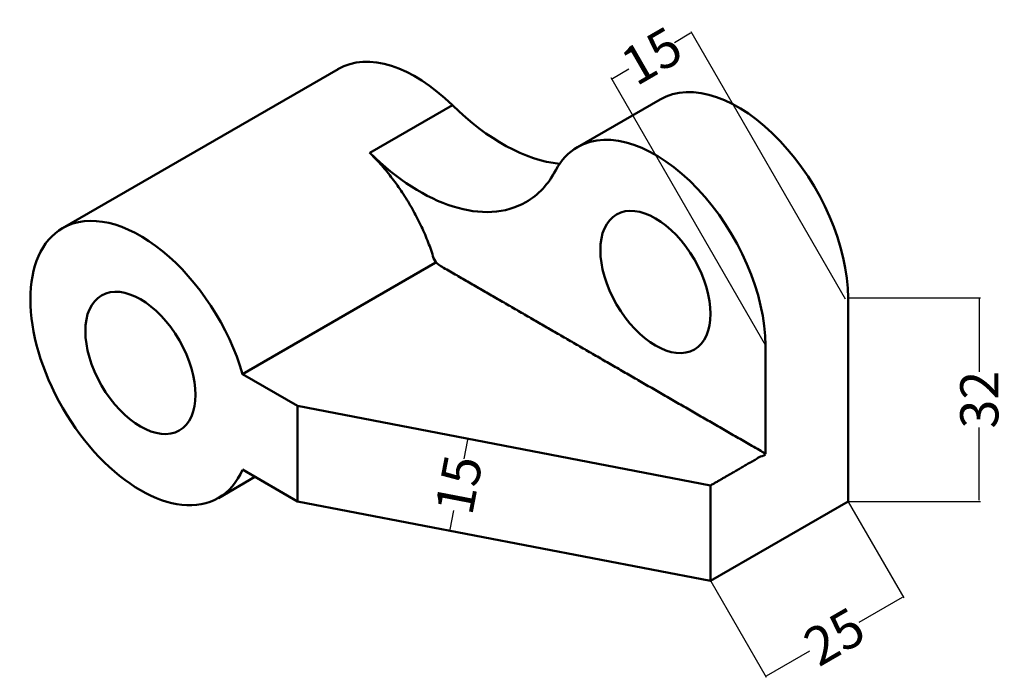
# Model space of a CAD drawing. Units: millimetres. Extents: x -32 to 123, y 29 to 132.
import ezdxf

# ---------------------------------------------------------------- set-up
doc = ezdxf.new("R2010")
doc.units = ezdxf.units.MM
doc.header["$MEASUREMENT"] = 0
doc.layers.add('M-DIMS', color=2, linetype='Continuous', lineweight=25)
doc.layers.add('M-OUTL', color=7, linetype='Continuous', lineweight=50)
doc.styles.get("Standard").update_dxf_attribs({"font": 'arial.ttf'})
doc.dimstyles.get("Standard").update_dxf_attribs({"dimtxt": 6, "dimasz": 0.18, "dimexe": 0.18, "dimexo": 0.0625, "dimgap": 0.09, "dimtad": 0, "dimtoh": 1, "dimdec": 0, "dimzin": 0, "dimdsep": 46, "dimtxsty": 'Standard', "dimcen": 0.09, "dimadec": 0, "dimazin": 0, "dimtfac": 1, "dimtdec": 0, "dimtofl": 0, "dimtmove": 0, "dimatfit": 3, "dimfxl": 1, "dimtolj": 1, "dimtzin": 0, "dimarcsym": 0})

# ---------------------------------------------------------------- blocks, each defined once
blk = doc.blocks.new('*D1')
at = {"layer": 'Defpoints', "color": 0, "transparency": 16777216}
for p in [(43.86, 65.27), (35.35, 51.9), (41.08, 50.8)]:
    blk.add_point(p, dxfattribs=at)
at = {"layer": 'M-DIMS', "color": 0, "lineweight": -2, "transparency": 16777216}
for p, q in [((38.1, 66.19), (37.52, 63.19)), ((43.8, 65.28), (37.96, 66.4)), ((35.38, 52.08), (35.96, 55.08)), ((41.02, 50.81), (35.17, 51.94))]:
    blk.add_line(p, q, dxfattribs=at)
at = {"layer": 'M-DIMS', "color": 0, "transparency": 16777216}
for points in [[(38.07, 66.2), (38.13, 66.19), (38.13, 66.37)], [(35.35, 52.09), (35.41, 52.08), (35.35, 51.9)]]:
    blk.add_solid(points, dxfattribs=at)
at = {"layer": 'M-DIMS', "color": 0, "transparency": 16777216, "insert": (36.74, 59.14), "char_height": 6, "attachment_point": 5, "rotation": 79.1066}
blk.add_mtext('\\A1;15', dxfattribs=at)
blk = doc.blocks.new('*D2')
at = {"layer": 'Defpoints', "color": 0, "transparency": 16777216}
for p in [(97.99, 56.52), (76.34, 44.02), (106.65, 41.52)]:
    blk.add_point(p, dxfattribs=at)
at = {"layer": 'M-DIMS', "color": 0, "lineweight": -2, "transparency": 16777216}
for p, q in [((98.02, 56.46), (106.74, 41.36)), ((76.37, 43.96), (85.09, 28.86)), ((106.49, 41.43), (99.68, 37.5)), ((85.15, 29.11), (91.96, 33.04))]:
    blk.add_line(p, q, dxfattribs=at)
at = {"layer": 'M-DIMS', "color": 0, "transparency": 16777216}
for points in [[(106.48, 41.45), (106.51, 41.4), (106.65, 41.52)], [(85.14, 29.13), (85.17, 29.08), (85, 29.02)]]:
    blk.add_solid(points, dxfattribs=at)
at = {"layer": 'M-DIMS', "color": 0, "transparency": 16777216, "insert": (95.82, 35.27), "char_height": 6, "attachment_point": 5, "rotation": 30}
blk.add_mtext('\\A1;25', dxfattribs=at)
blk = doc.blocks.new('*D3')
at = {"layer": 'Defpoints', "color": 0, "transparency": 16777216}
for p in [(97.99, 88.52), (97.99, 56.52), (118.62, 56.52)]:
    blk.add_point(p, dxfattribs=at)
at = {"layer": 'M-DIMS', "color": 0, "lineweight": -2, "transparency": 16777216}
for p, q in [((98.05, 88.52), (118.8, 88.52)), ((118.62, 88.34), (118.62, 76.87)), ((118.62, 56.7), (118.62, 68.16)), ((98.05, 56.52), (118.8, 56.52))]:
    blk.add_line(p, q, dxfattribs=at)
at = {"layer": 'M-DIMS', "color": 0, "transparency": 16777216}
for points in [[(118.59, 88.34), (118.65, 88.34), (118.62, 88.52)], [(118.59, 56.7), (118.65, 56.7), (118.62, 56.52)]]:
    blk.add_solid(points, dxfattribs=at)
at = {"layer": 'M-DIMS', "color": 0, "transparency": 16777216, "insert": (118.62, 72.52), "char_height": 6, "attachment_point": 5, "rotation": 90}
blk.add_mtext('\\A1;32', dxfattribs=at)
blk = doc.blocks.new('*D4')
at = {"layer": 'Defpoints', "color": 0, "transparency": 16777216}
for p in [(73.38, 130.2), (97.58, 88.28), (85, 81.02)]:
    blk.add_point(p, dxfattribs=at)
at = {"layer": 'M-DIMS', "color": 0, "lineweight": -2, "transparency": 16777216}
for p, q in [((73.22, 130.11), (70.66, 128.63)), ((97.55, 88.33), (73.29, 130.36)), ((60.95, 123.03), (63.51, 124.51)), ((84.97, 81.07), (60.7, 123.09))]:
    blk.add_line(p, q, dxfattribs=at)
at = {"layer": 'M-DIMS', "color": 0, "transparency": 16777216}
for points in [[(73.2, 130.14), (73.23, 130.09), (73.38, 130.2)], [(60.93, 123.05), (60.96, 123), (60.79, 122.94)]]:
    blk.add_solid(points, dxfattribs=at)
at = {"layer": 'M-DIMS', "color": 0, "transparency": 16777216, "insert": (67.08, 126.57), "char_height": 6, "attachment_point": 5, "rotation": 30}
blk.add_mtext('\\A1;15', dxfattribs=at)

msp = doc.modelspace()

# ---------------------------------------------------------------- linework, layer by layer
at = {"layer": 'M-OUTL'}
for p, q in [((-25.56, 99.48), (17.75, 124.48)), ((55.42, 112.23), (68.41, 119.73)), ((22.77, 111.3), (35.76, 118.8)), ((84.99, 64.02), (84.99, 81.02)), ((-1.06, 57.05), (4.69, 60.38))]:
    msp.add_line(p, q, dxfattribs=at)
for points in [[(11.38, 71.52), (2.72, 76.52), (33.04, 94.02)], [(76.34, 44.02), (97.99, 56.52), (97.99, 88.52)], [(11.38, 56.52), (76.34, 44.02), (76.34, 59.02), (11.38, 71.52), (11.38, 56.52), (2.72, 61.52)]]:
    msp.add_lwpolyline(points, dxfattribs=at)
for centre, major_axis, start_param, end_param in [((29.99, 103.27), (12.25, -21.21), 2.01693, 3.141593), ((80.66, 98.52), (-12.25, 21.21), 3.926991, 6.283185), ((43.58, 140.04), (16.72, -28.96), 5.160393, 5.889516), ((67.67, 91.02), (-12.25, 21.21), 3.926991, 6.283185), ((67.67, 91.02), (-12.25, 21.21), 0, 0.345139), ((30.59, 132.54), (16.72, -28.96), 5.160393, 6.283185), ((30.59, 132.54), (16.72, -28.96), 0, 0.346645), ((-13.31, 78.27), (12.25, -21.21), 1.169795, 3.141593), ((-13.31, 78.27), (12.25, -21.21), 3.141593, 6.283185), ((-13.31, 78.27), (12.25, -21.21), 0, 0.401001)]:
    msp.add_ellipse(centre, major_axis=major_axis, ratio=0.57735, start_param=start_param, end_param=end_param, dxfattribs=at)
for centre in [(67.68, 91.02), (-13.33, 78.29)]:
    msp.add_ellipse(centre, major_axis=(6.12, -10.61), ratio=0.57735, dxfattribs=at)
msp.add_rational_spline([(76.34, 59.02), (80.67, 61.52), (85, 64.02), (71.77, 71.65), (58.55, 79.28), (45.79, 86.65), (33.04, 94.02), (30.1, 104.11), (22.69, 111.37)], [1, 1, 1, 1, 1, 1, 1, 0.910998186126, 1], degree=2, knots=[0, 0, 0, 1, 1, 2, 2, 3, 3, 3.850197, 3.850197, 3.850197], dxfattribs=at)

# ---------------------------------------------------------------- dimensions: what is measured, and where the dimension line sits
at = {"layer": 'M-DIMS'}
for p1, p2, distance, picture, middle in [((85, 81.02), (97.58, 88.28), 48.41, '*D4', (67.08, 126.57)), ((97.99, 88.52), (97.99, 56.52), 20.63, '*D3', (118.62, 72.52)), ((43.86, 65.27), (41.08, 50.8), -5.83, '*D1', (36.74, 59.14)), ((76.34, 44.02), (97.99, 56.52), -17.32, '*D2', (95.82, 35.27))]:
    dim = msp.add_aligned_dim(p1=p1, p2=p2, distance=distance, dimstyle='Standard', override={"dimclrd": 0, "dimclre": 0, "dimclrt": 0}, dxfattribs=at)
    dim.commit()
    dim.dimension.update_dxf_attribs({"geometry": picture, "text_midpoint": middle})

doc.saveas('drawing.dxf')
